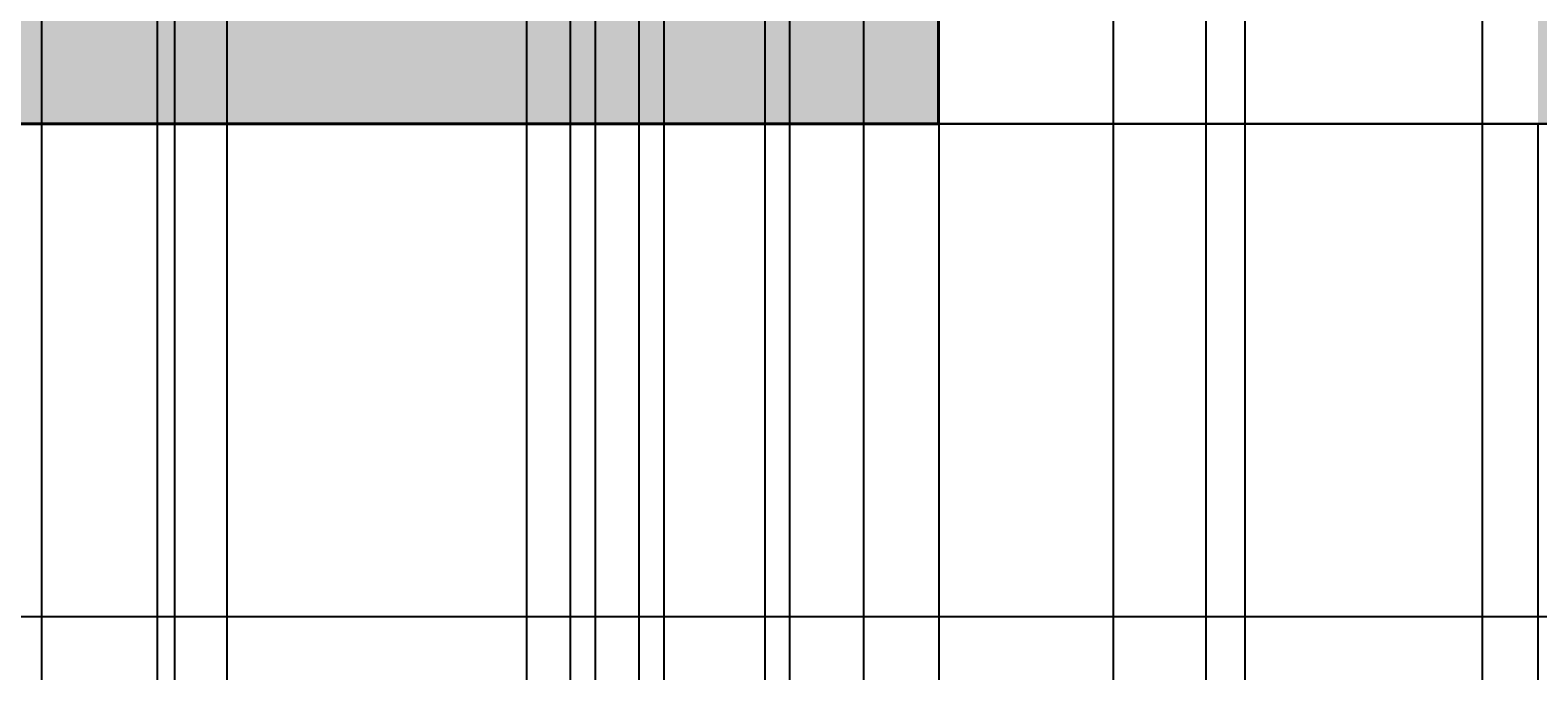
# Model space of a CAD drawing. Units: inches. Extents: x 818 to 1898, y 976 to 2364.
# Tile 35 of 96: x 1391 to 1512, y 1643 to 1695. Entities that reach past the tile are written whole.
import ezdxf

# ---------------------------------------------------------------- set-up
doc = ezdxf.new("R2010")
doc.units = ezdxf.units.IN
doc.header["$LTSCALE"] = 5
doc.header["$MEASUREMENT"] = 0
doc.layers.add('A-ANNO-DIMS', color=2, linetype='Continuous', lineweight=18)
doc.layers.add('A-WALL', color=7, linetype='Continuous', lineweight=40)
doc.layers.add('A-WALL-PATT', color=251, linetype='Continuous', lineweight=13, true_color=0x636466)
doc.styles.get("Standard").update_dxf_attribs({"font": 'arial.ttf'})
doc.dimstyles.get("Standard").update_dxf_attribs({"dimtxt": 0.18, "dimasz": 0.18, "dimexe": 0.18, "dimexo": 0.0625, "dimgap": 0.09, "dimtad": 0, "dimtih": 1, "dimtoh": 1, "dimdec": 4, "dimzin": 0, "dimdsep": 46, "dimtxsty": 'Standard', "dimcen": 0.09, "dimadec": 0, "dimazin": 0, "dimtfac": 1, "dimtdec": 4, "dimtofl": 0, "dimtmove": 0, "dimatfit": 3, "dimfxl": 1, "dimtolj": 1, "dimtzin": 0, "dimarcsym": 0})

# ---------------------------------------------------------------- blocks, each defined once
blk = doc.blocks.new('*D61')
at = {"layer": 'A-ANNO-DIMS', "color": 0, "lineweight": -2, "ltscale": 5, "transparency": 16777216}
for p, q in [((1071.73, 1203.03), (1071.73, 2363.87)), ((1071.91, 2363.69), (1250.94, 2363.69)), ((1430.55, 2363.69), (1251.51, 2363.69)), ((1430.73, 1203.03), (1430.73, 2363.87))]:
    blk.add_line(p, q, dxfattribs=at)
at = {"layer": 'A-ANNO-DIMS', "color": 0, "ltscale": 5, "transparency": 16777216}
for points in [[(1071.91, 2363.72), (1071.91, 2363.66), (1071.73, 2363.69)], [(1430.55, 2363.72), (1430.55, 2363.66), (1430.73, 2363.69)]]:
    blk.add_solid(points, dxfattribs=at)
at = {"layer": 'Defpoints', "color": 0, "ltscale": 5, "transparency": 16777216}
for p in [(1430.73, 2363.69), (1071.73, 1202.96), (1430.73, 1202.96)]:
    blk.add_point(p, dxfattribs=at)
at = {"layer": 'A-ANNO-DIMS', "color": 0, "ltscale": 5, "transparency": 16777216, "insert": (1251.23, 2363.69), "char_height": 0.18, "attachment_point": 5}
blk.add_mtext('\\A1;359', dxfattribs=at)
blk = doc.blocks.new('*D64')
at = {"layer": 'A-ANNO-DIMS', "color": 0, "lineweight": -2, "ltscale": 5, "transparency": 16777216}
for p, q in [((1197.73, 1501.14), (1197.73, 2363.87)), ((1197.91, 2363.69), (1313.93, 2363.69)), ((1430.55, 2363.69), (1314.52, 2363.69)), ((1430.73, 1501.14), (1430.73, 2363.87))]:
    blk.add_line(p, q, dxfattribs=at)
at = {"layer": 'A-ANNO-DIMS', "color": 0, "ltscale": 5, "transparency": 16777216}
for points in [[(1197.91, 2363.72), (1197.91, 2363.66), (1197.73, 2363.69)], [(1430.55, 2363.72), (1430.55, 2363.66), (1430.73, 2363.69)]]:
    blk.add_solid(points, dxfattribs=at)
at = {"layer": 'Defpoints', "color": 0, "ltscale": 5, "transparency": 16777216}
for p in [(1430.73, 2363.69), (1197.73, 1501.08), (1430.73, 1501.08)]:
    blk.add_point(p, dxfattribs=at)
at = {"layer": 'A-ANNO-DIMS', "color": 0, "ltscale": 5, "transparency": 16777216, "insert": (1314.23, 2363.69), "char_height": 0.18, "attachment_point": 5}
blk.add_mtext('\\A1;233', dxfattribs=at)
blk = doc.blocks.new('*D98')
at = {"layer": 'A-ANNO-DIMS', "color": 0, "lineweight": -2, "ltscale": 5, "transparency": 16777216}
for p, q in [((1338.54, 1071.12), (1338.54, 2363.87)), ((1338.72, 2363.69), (1364.81, 2363.69)), ((1391.7, 2363.69), (1365.6, 2363.69)), ((1391.88, 1071.12), (1391.88, 2363.87))]:
    blk.add_line(p, q, dxfattribs=at)
at = {"layer": 'A-ANNO-DIMS', "color": 0, "ltscale": 5, "transparency": 16777216}
for points in [[(1338.72, 2363.72), (1338.72, 2363.66), (1338.54, 2363.69)], [(1391.7, 2363.72), (1391.7, 2363.66), (1391.88, 2363.69)]]:
    blk.add_solid(points, dxfattribs=at)
at = {"layer": 'Defpoints', "color": 0, "ltscale": 5, "transparency": 16777216}
for p in [(1391.88, 2363.69), (1338.54, 1071.06), (1391.88, 1071.06)]:
    blk.add_point(p, dxfattribs=at)
at = {"layer": 'A-ANNO-DIMS', "color": 0, "ltscale": 5, "transparency": 16777216, "insert": (1365.21, 2363.69), "char_height": 0.18, "attachment_point": 5}
blk.add_mtext('\\A1;53.33', dxfattribs=at)
blk = doc.blocks.new('*D99')
at = {"layer": 'A-ANNO-DIMS', "color": 0, "lineweight": -2, "ltscale": 5, "transparency": 16777216}
for p, q in [((1391.88, 1071.12), (1391.88, 2363.87)), ((1392.06, 2363.69), (1420.45, 2363.69)), ((1449.64, 2363.69), (1421.24, 2363.69)), ((1449.82, 1071.12), (1449.82, 2363.87))]:
    blk.add_line(p, q, dxfattribs=at)
at = {"layer": 'A-ANNO-DIMS', "color": 0, "ltscale": 5, "transparency": 16777216}
for points in [[(1392.06, 2363.72), (1392.06, 2363.66), (1391.88, 2363.69)], [(1449.64, 2363.72), (1449.64, 2363.66), (1449.82, 2363.69)]]:
    blk.add_solid(points, dxfattribs=at)
at = {"layer": 'Defpoints', "color": 0, "ltscale": 5, "transparency": 16777216}
for p in [(1449.82, 2363.69), (1391.88, 1071.06), (1449.82, 1071.06)]:
    blk.add_point(p, dxfattribs=at)
at = {"layer": 'A-ANNO-DIMS', "color": 0, "ltscale": 5, "transparency": 16777216, "insert": (1420.85, 2363.69), "char_height": 0.18, "attachment_point": 5}
blk.add_mtext('\\A1;57.94', dxfattribs=at)
blk = doc.blocks.new('*D100')
at = {"layer": 'A-ANNO-DIMS', "color": 0, "lineweight": -2, "ltscale": 5, "transparency": 16777216}
for p, q in [((1449.82, 1071.12), (1449.82, 2363.87)), ((1450, 2363.69), (1478.17, 2363.69)), ((1507.12, 2363.69), (1478.95, 2363.69)), ((1507.3, 1071.12), (1507.3, 2363.87))]:
    blk.add_line(p, q, dxfattribs=at)
at = {"layer": 'A-ANNO-DIMS', "color": 0, "ltscale": 5, "transparency": 16777216}
for points in [[(1450, 2363.72), (1450, 2363.66), (1449.82, 2363.69)], [(1507.12, 2363.72), (1507.12, 2363.66), (1507.3, 2363.69)]]:
    blk.add_solid(points, dxfattribs=at)
at = {"layer": 'Defpoints', "color": 0, "ltscale": 5, "transparency": 16777216}
for p in [(1507.3, 2363.69), (1449.82, 1071.06), (1507.3, 1071.06)]:
    blk.add_point(p, dxfattribs=at)
at = {"layer": 'A-ANNO-DIMS', "color": 0, "ltscale": 5, "transparency": 16777216, "insert": (1478.56, 2363.69), "char_height": 0.18, "attachment_point": 5}
blk.add_mtext('\\A1;57.48', dxfattribs=at)
blk = doc.blocks.new('*D101')
at = {"layer": 'A-ANNO-DIMS', "color": 0, "lineweight": -2, "ltscale": 5, "transparency": 16777216}
for p, q in [((1507.3, 1071.12), (1507.3, 2363.87)), ((1507.48, 2363.69), (1536, 2363.69)), ((1565.3, 2363.69), (1536.78, 2363.69)), ((1565.48, 1071.12), (1565.48, 2363.87))]:
    blk.add_line(p, q, dxfattribs=at)
at = {"layer": 'A-ANNO-DIMS', "color": 0, "ltscale": 5, "transparency": 16777216}
for points in [[(1507.48, 2363.72), (1507.48, 2363.66), (1507.3, 2363.69)], [(1565.3, 2363.72), (1565.3, 2363.66), (1565.48, 2363.69)]]:
    blk.add_solid(points, dxfattribs=at)
at = {"layer": 'Defpoints', "color": 0, "ltscale": 5, "transparency": 16777216}
for p in [(1565.48, 2363.69), (1507.3, 1071.06), (1565.48, 1071.06)]:
    blk.add_point(p, dxfattribs=at)
at = {"layer": 'A-ANNO-DIMS', "color": 0, "ltscale": 5, "transparency": 16777216, "insert": (1536.39, 2363.69), "char_height": 0.18, "attachment_point": 5}
blk.add_mtext('\\A1;58.19', dxfattribs=at)
blk = doc.blocks.new('*D119')
at = {"layer": 'A-ANNO-DIMS', "color": 0, "lineweight": -2, "ltscale": 5, "transparency": 16777216}
for p, q in [((1766.29, 1716.99), (818.03, 1716.99)), ((818.21, 1716.81), (818.21, 1672.43)), ((818.21, 1627.69), (818.21, 1672.06)), ((1766.29, 1627.51), (818.03, 1627.51))]:
    blk.add_line(p, q, dxfattribs=at)
at = {"layer": 'A-ANNO-DIMS', "color": 0, "ltscale": 5, "transparency": 16777216}
for points in [[(818.18, 1716.81), (818.24, 1716.81), (818.21, 1716.99)], [(818.18, 1627.69), (818.24, 1627.69), (818.21, 1627.51)]]:
    blk.add_solid(points, dxfattribs=at)
at = {"layer": 'Defpoints', "color": 0, "ltscale": 5, "transparency": 16777216}
for p in [(818.21, 1716.99), (1766.35, 1716.99), (1766.35, 1627.51)]:
    blk.add_point(p, dxfattribs=at)
at = {"layer": 'A-ANNO-DIMS', "color": 0, "ltscale": 5, "transparency": 16777216, "insert": (818.21, 1672.25), "char_height": 0.18, "attachment_point": 5}
blk.add_mtext('\\A1;89.48', dxfattribs=at)
blk = doc.blocks.new('*D159')
at = {"layer": 'A-ANNO-DIMS', "color": 0, "lineweight": -2, "ltscale": 5, "transparency": 16777216}
for p, q in [((1206.73, 1687.02), (1206.73, 975.66)), ((1463.73, 1687.02), (1463.73, 975.66)), ((1206.91, 975.84), (1334.93, 975.84)), ((1463.55, 975.84), (1335.52, 975.84))]:
    blk.add_line(p, q, dxfattribs=at)
at = {"layer": 'A-ANNO-DIMS', "color": 0, "ltscale": 5, "transparency": 16777216}
for points in [[(1206.91, 975.87), (1206.91, 975.81), (1206.73, 975.84)], [(1463.55, 975.87), (1463.55, 975.81), (1463.73, 975.84)]]:
    blk.add_solid(points, dxfattribs=at)
at = {"layer": 'Defpoints', "color": 0, "ltscale": 5, "transparency": 16777216}
for p in [(1206.73, 1687.08), (1463.73, 1687.08), (1463.73, 975.84)]:
    blk.add_point(p, dxfattribs=at)
at = {"layer": 'A-ANNO-DIMS', "color": 0, "ltscale": 5, "transparency": 16777216, "insert": (1335.23, 975.84), "char_height": 0.18, "attachment_point": 5}
blk.add_mtext('\\A1;257', dxfattribs=at)
blk = doc.blocks.new('*D160')
at = {"layer": 'A-ANNO-DIMS', "color": 0, "lineweight": -2, "ltscale": 5, "transparency": 16777216}
for p, q in [((1463.73, 1687.02), (1463.73, 975.66)), ((1511.73, 1687.02), (1511.73, 975.66)), ((1463.91, 975.84), (1487.5, 975.84)), ((1511.55, 975.84), (1487.95, 975.84))]:
    blk.add_line(p, q, dxfattribs=at)
at = {"layer": 'A-ANNO-DIMS', "color": 0, "ltscale": 5, "transparency": 16777216}
for points in [[(1463.91, 975.87), (1463.91, 975.81), (1463.73, 975.84)], [(1511.55, 975.87), (1511.55, 975.81), (1511.73, 975.84)]]:
    blk.add_solid(points, dxfattribs=at)
at = {"layer": 'Defpoints', "color": 0, "ltscale": 5, "transparency": 16777216}
for p in [(1463.73, 1687.08), (1511.73, 1687.08), (1511.73, 975.84)]:
    blk.add_point(p, dxfattribs=at)
at = {"layer": 'A-ANNO-DIMS', "color": 0, "ltscale": 5, "transparency": 16777216, "insert": (1487.73, 975.84), "char_height": 0.18, "attachment_point": 5}
blk.add_mtext('\\A1;48', dxfattribs=at)
blk = doc.blocks.new('*D166')
at = {"layer": 'A-ANNO-DIMS', "color": 0, "lineweight": -2, "ltscale": 5, "transparency": 16777216}
for p, q in [((1401.15, 1510.14), (1401.15, 2363.87)), ((1401.33, 2363.69), (1415.54, 2363.69)), ((1430.55, 2363.69), (1416.33, 2363.69)), ((1430.73, 1510.14), (1430.73, 2363.87))]:
    blk.add_line(p, q, dxfattribs=at)
at = {"layer": 'A-ANNO-DIMS', "color": 0, "ltscale": 5, "transparency": 16777216}
for points in [[(1401.33, 2363.72), (1401.33, 2363.66), (1401.15, 2363.69)], [(1430.55, 2363.72), (1430.55, 2363.66), (1430.73, 2363.69)]]:
    blk.add_solid(points, dxfattribs=at)
at = {"layer": 'Defpoints', "color": 0, "ltscale": 5, "transparency": 16777216}
for p in [(1430.73, 2363.69), (1401.15, 1510.08), (1430.73, 1510.08)]:
    blk.add_point(p, dxfattribs=at)
at = {"layer": 'A-ANNO-DIMS', "color": 0, "ltscale": 5, "transparency": 16777216, "insert": (1415.94, 2363.69), "char_height": 0.18, "attachment_point": 5}
blk.add_mtext('\\A1;29.58', dxfattribs=at)
blk = doc.blocks.new('*D169')
at = {"layer": 'A-ANNO-DIMS', "color": 0, "lineweight": -2, "ltscale": 5, "transparency": 16777216}
for p, q in [((1441.73, 1600.14), (1441.73, 2363.87)), ((1441.91, 2363.69), (1459.51, 2363.69)), ((1477.55, 2363.69), (1459.94, 2363.69)), ((1477.73, 1600.14), (1477.73, 2363.87))]:
    blk.add_line(p, q, dxfattribs=at)
at = {"layer": 'A-ANNO-DIMS', "color": 0, "ltscale": 5, "transparency": 16777216}
for points in [[(1441.91, 2363.72), (1441.91, 2363.66), (1441.73, 2363.69)], [(1477.55, 2363.72), (1477.55, 2363.66), (1477.73, 2363.69)]]:
    blk.add_solid(points, dxfattribs=at)
at = {"layer": 'Defpoints', "color": 0, "ltscale": 5, "transparency": 16777216}
for p in [(1477.73, 2363.69), (1441.73, 1600.08), (1477.73, 1600.08)]:
    blk.add_point(p, dxfattribs=at)
at = {"layer": 'A-ANNO-DIMS', "color": 0, "ltscale": 5, "transparency": 16777216, "insert": (1459.73, 2363.69), "char_height": 0.18, "attachment_point": 5}
blk.add_mtext('\\A1;36', dxfattribs=at)
blk = doc.blocks.new('*D176')
at = {"layer": 'A-ANNO-DIMS', "color": 0, "lineweight": -2, "ltscale": 5, "transparency": 16777216}
for p, q in [((1559.66, 1687.08), (818.03, 1687.08)), ((818.21, 1686.9), (818.21, 1667.51)), ((818.21, 1647.76), (818.21, 1667.15)), ((1559.66, 1647.58), (818.03, 1647.58))]:
    blk.add_line(p, q, dxfattribs=at)
at = {"layer": 'A-ANNO-DIMS', "color": 0, "ltscale": 5, "transparency": 16777216}
for points in [[(818.18, 1686.9), (818.24, 1686.9), (818.21, 1687.08)], [(818.18, 1647.76), (818.24, 1647.76), (818.21, 1647.58)]]:
    blk.add_solid(points, dxfattribs=at)
at = {"layer": 'Defpoints', "color": 0, "ltscale": 5, "transparency": 16777216}
for p in [(1559.73, 1687.08), (818.21, 1647.58), (1559.73, 1647.58)]:
    blk.add_point(p, dxfattribs=at)
at = {"layer": 'A-ANNO-DIMS', "color": 0, "ltscale": 5, "transparency": 16777216, "insert": (818.21, 1667.33), "char_height": 0.18, "attachment_point": 5}
blk.add_mtext('\\A1;39.5', dxfattribs=at)
blk = doc.blocks.new('*D182')
at = {"layer": 'A-ANNO-DIMS', "color": 0, "lineweight": -2, "ltscale": 5, "transparency": 16777216}
for p, q in [((1463.73, 1687.02), (1463.73, 975.66)), ((1559.73, 1687.02), (1559.73, 975.66)), ((1463.91, 975.84), (1511.51, 975.84)), ((1559.55, 975.84), (1511.94, 975.84))]:
    blk.add_line(p, q, dxfattribs=at)
at = {"layer": 'A-ANNO-DIMS', "color": 0, "ltscale": 5, "transparency": 16777216}
for points in [[(1463.91, 975.87), (1463.91, 975.81), (1463.73, 975.84)], [(1559.55, 975.87), (1559.55, 975.81), (1559.73, 975.84)]]:
    blk.add_solid(points, dxfattribs=at)
at = {"layer": 'Defpoints', "color": 0, "ltscale": 5, "transparency": 16777216}
for p in [(1463.73, 1687.08), (1559.73, 1687.08), (1559.73, 975.84)]:
    blk.add_point(p, dxfattribs=at)
at = {"layer": 'A-ANNO-DIMS', "color": 0, "ltscale": 5, "transparency": 16777216, "insert": (1511.73, 975.84), "char_height": 0.18, "attachment_point": 5}
blk.add_mtext('\\A1;96', dxfattribs=at)
blk = doc.blocks.new('*D191')
at = {"layer": 'A-ANNO-DIMS', "color": 0, "lineweight": -2, "ltscale": 5, "transparency": 16777216}
for p, q in [((1434.23, 1409.11), (1434.23, 2363.87)), ((1434.41, 2363.69), (1435.08, 2363.69)), ((1436.05, 2363.69), (1435.37, 2363.69)), ((1436.23, 1409.11), (1436.23, 2363.87))]:
    blk.add_line(p, q, dxfattribs=at)
at = {"layer": 'A-ANNO-DIMS', "color": 0, "ltscale": 5, "transparency": 16777216}
for points in [[(1434.41, 2363.72), (1434.41, 2363.66), (1434.23, 2363.69)], [(1436.05, 2363.72), (1436.05, 2363.66), (1436.23, 2363.69)]]:
    blk.add_solid(points, dxfattribs=at)
at = {"layer": 'Defpoints', "color": 0, "ltscale": 5, "transparency": 16777216}
for p in [(1436.23, 2363.69), (1434.23, 1409.05), (1436.23, 1409.05)]:
    blk.add_point(p, dxfattribs=at)
at = {"layer": 'A-ANNO-DIMS', "color": 0, "ltscale": 5, "transparency": 16777216, "insert": (1435.23, 2363.69), "char_height": 0.18, "attachment_point": 5}
blk.add_mtext('\\A1;2', dxfattribs=at)
blk = doc.blocks.new('*D196')
at = {"layer": 'A-ANNO-DIMS', "color": 0, "lineweight": -2, "ltscale": 5, "transparency": 16777216}
for p, q in [((1439.73, 1526.73), (1439.73, 2363.87)), ((1439.91, 2363.69), (1448.51, 2363.69)), ((1457.55, 2363.69), (1448.94, 2363.69)), ((1457.73, 1526.73), (1457.73, 2363.87))]:
    blk.add_line(p, q, dxfattribs=at)
at = {"layer": 'A-ANNO-DIMS', "color": 0, "ltscale": 5, "transparency": 16777216}
for points in [[(1439.91, 2363.72), (1439.91, 2363.66), (1439.73, 2363.69)], [(1457.55, 2363.72), (1457.55, 2363.66), (1457.73, 2363.69)]]:
    blk.add_solid(points, dxfattribs=at)
at = {"layer": 'Defpoints', "color": 0, "ltscale": 5, "transparency": 16777216}
for p in [(1457.73, 2363.69), (1439.73, 1526.67), (1457.73, 1526.67)]:
    blk.add_point(p, dxfattribs=at)
at = {"layer": 'A-ANNO-DIMS', "color": 0, "ltscale": 5, "transparency": 16777216, "insert": (1448.73, 2363.69), "char_height": 0.18, "attachment_point": 5}
blk.add_mtext('\\A1;18', dxfattribs=at)
blk = doc.blocks.new('*D214')
at = {"layer": 'A-ANNO-DIMS', "color": 0, "lineweight": -2, "ltscale": 5, "transparency": 16777216}
for p, q in [((1511.73, 1687.02), (1511.73, 975.66)), ((1714.73, 1687.02), (1714.73, 975.66)), ((1511.91, 975.84), (1612.93, 975.84)), ((1714.55, 975.84), (1613.52, 975.84))]:
    blk.add_line(p, q, dxfattribs=at)
at = {"layer": 'A-ANNO-DIMS', "color": 0, "ltscale": 5, "transparency": 16777216}
for points in [[(1511.91, 975.87), (1511.91, 975.81), (1511.73, 975.84)], [(1714.55, 975.87), (1714.55, 975.81), (1714.73, 975.84)]]:
    blk.add_solid(points, dxfattribs=at)
at = {"layer": 'Defpoints', "color": 0, "ltscale": 5, "transparency": 16777216}
for p in [(1511.73, 1687.08), (1714.73, 1687.08), (1714.73, 975.84)]:
    blk.add_point(p, dxfattribs=at)
at = {"layer": 'A-ANNO-DIMS', "color": 0, "ltscale": 5, "transparency": 16777216, "insert": (1613.23, 975.84), "char_height": 0.18, "attachment_point": 5}
blk.add_mtext('\\A1;203', dxfattribs=at)
blk = doc.blocks.new('*D215')
at = {"layer": 'A-ANNO-DIMS', "color": 0, "lineweight": -2, "ltscale": 5, "transparency": 16777216}
for p, q in [((1590.66, 1876.08), (818.03, 1876.08)), ((818.21, 1875.9), (818.21, 1781.76)), ((818.21, 1687.26), (818.21, 1781.4)), ((1511.66, 1687.08), (818.03, 1687.08))]:
    blk.add_line(p, q, dxfattribs=at)
at = {"layer": 'A-ANNO-DIMS', "color": 0, "ltscale": 5, "transparency": 16777216}
for points in [[(818.18, 1875.9), (818.24, 1875.9), (818.21, 1876.08)], [(818.18, 1687.26), (818.24, 1687.26), (818.21, 1687.08)]]:
    blk.add_solid(points, dxfattribs=at)
at = {"layer": 'Defpoints', "color": 0, "ltscale": 5, "transparency": 16777216}
for p in [(818.21, 1876.08), (1590.73, 1876.08), (1511.73, 1687.08)]:
    blk.add_point(p, dxfattribs=at)
at = {"layer": 'A-ANNO-DIMS', "color": 0, "ltscale": 5, "transparency": 16777216, "insert": (818.21, 1781.58), "char_height": 0.18, "attachment_point": 5}
blk.add_mtext('\\A1;189', dxfattribs=at)
blk = doc.blocks.new('*D231')
at = {"layer": 'A-ANNO-DIMS', "color": 0, "lineweight": -2, "ltscale": 5, "transparency": 16777216}
for p, q in [((1303.93, 1952.98), (1303.93, 975.66)), ((1402.52, 1952.98), (1402.52, 975.66)), ((1304.11, 975.84), (1352.83, 975.84)), ((1402.34, 975.84), (1353.62, 975.84))]:
    blk.add_line(p, q, dxfattribs=at)
at = {"layer": 'A-ANNO-DIMS', "color": 0, "ltscale": 5, "transparency": 16777216}
for points in [[(1304.11, 975.87), (1304.11, 975.81), (1303.93, 975.84)], [(1402.34, 975.87), (1402.34, 975.81), (1402.52, 975.84)]]:
    blk.add_solid(points, dxfattribs=at)
at = {"layer": 'Defpoints', "color": 0, "ltscale": 5, "transparency": 16777216}
for p in [(1303.93, 1953.04), (1402.52, 1953.04), (1402.52, 975.84)]:
    blk.add_point(p, dxfattribs=at)
at = {"layer": 'A-ANNO-DIMS', "color": 0, "ltscale": 5, "transparency": 16777216, "insert": (1353.22, 975.84), "char_height": 0.18, "attachment_point": 5}
blk.add_mtext('\\A1;98.59', dxfattribs=at)
blk = doc.blocks.new('*D242')
at = {"layer": 'A-ANNO-DIMS', "color": 0, "lineweight": -2, "ltscale": 5, "transparency": 16777216}
for p, q in [((1488.26, 1948.6), (1488.26, 975.66)), ((1513.23, 1948.6), (1513.23, 975.66)), ((1488.44, 975.84), (1500.35, 975.84)), ((1513.05, 975.84), (1501.14, 975.84))]:
    blk.add_line(p, q, dxfattribs=at)
at = {"layer": 'A-ANNO-DIMS', "color": 0, "ltscale": 5, "transparency": 16777216}
for points in [[(1488.44, 975.87), (1488.44, 975.81), (1488.26, 975.84)], [(1513.05, 975.87), (1513.05, 975.81), (1513.23, 975.84)]]:
    blk.add_solid(points, dxfattribs=at)
at = {"layer": 'Defpoints', "color": 0, "ltscale": 5, "transparency": 16777216}
for p in [(1488.26, 1948.66), (1513.23, 1948.66), (1513.23, 975.84)]:
    blk.add_point(p, dxfattribs=at)
at = {"layer": 'A-ANNO-DIMS', "color": 0, "ltscale": 5, "transparency": 16777216, "insert": (1500.74, 975.84), "char_height": 0.18, "attachment_point": 5}
blk.add_mtext('\\A1;24.97', dxfattribs=at)
blk = doc.blocks.new('*D243')
at = {"layer": 'A-ANNO-DIMS', "color": 0, "lineweight": -2, "ltscale": 5, "transparency": 16777216}
for p, q in [((1451.77, 2020.02), (1451.77, 975.66)), ((1590.73, 2020.02), (1590.73, 975.66)), ((1451.95, 975.84), (1520.79, 975.84)), ((1590.55, 975.84), (1521.7, 975.84))]:
    blk.add_line(p, q, dxfattribs=at)
at = {"layer": 'A-ANNO-DIMS', "color": 0, "ltscale": 5, "transparency": 16777216}
for points in [[(1451.95, 975.87), (1451.95, 975.81), (1451.77, 975.84)], [(1590.55, 975.87), (1590.55, 975.81), (1590.73, 975.84)]]:
    blk.add_solid(points, dxfattribs=at)
at = {"layer": 'Defpoints', "color": 0, "ltscale": 5, "transparency": 16777216}
for p in [(1451.77, 2020.08), (1590.73, 2020.08), (1590.73, 975.84)]:
    blk.add_point(p, dxfattribs=at)
at = {"layer": 'A-ANNO-DIMS', "color": 0, "ltscale": 5, "transparency": 16777216, "insert": (1521.25, 975.84), "char_height": 0.18, "attachment_point": 5}
blk.add_mtext('\\A1;138.96', dxfattribs=at)
blk = doc.blocks.new('*D253')
at = {"layer": 'A-ANNO-DIMS', "color": 0, "lineweight": -2, "ltscale": 5, "transparency": 16777216}
for p, q in [((1485.12, 2053.02), (1485.12, 975.66)), ((1538.52, 2053.02), (1538.52, 975.66)), ((1485.3, 975.84), (1511.42, 975.84)), ((1538.34, 975.84), (1512.21, 975.84))]:
    blk.add_line(p, q, dxfattribs=at)
at = {"layer": 'A-ANNO-DIMS', "color": 0, "ltscale": 5, "transparency": 16777216}
for points in [[(1485.3, 975.87), (1485.3, 975.81), (1485.12, 975.84)], [(1538.34, 975.87), (1538.34, 975.81), (1538.52, 975.84)]]:
    blk.add_solid(points, dxfattribs=at)
at = {"layer": 'Defpoints', "color": 0, "ltscale": 5, "transparency": 16777216}
for p in [(1485.12, 2053.08), (1538.52, 2053.08), (1538.52, 975.84)]:
    blk.add_point(p, dxfattribs=at)
at = {"layer": 'A-ANNO-DIMS', "color": 0, "ltscale": 5, "transparency": 16777216, "insert": (1511.82, 975.84), "char_height": 0.18, "attachment_point": 5}
blk.add_mtext('\\A1;53.39', dxfattribs=at)
blk = doc.blocks.new('*D273')
at = {"layer": 'A-ANNO-DIMS', "color": 0, "lineweight": -2, "ltscale": 5, "transparency": 16777216}
for p, q in [((1406.73, 1587.48), (1406.73, 2363.87)), ((1406.91, 2363.69), (1418.51, 2363.69)), ((1430.55, 2363.69), (1418.95, 2363.69)), ((1430.73, 1587.48), (1430.73, 2363.87))]:
    blk.add_line(p, q, dxfattribs=at)
at = {"layer": 'A-ANNO-DIMS', "color": 0, "ltscale": 5, "transparency": 16777216}
for points in [[(1406.91, 2363.72), (1406.91, 2363.66), (1406.73, 2363.69)], [(1430.55, 2363.72), (1430.55, 2363.66), (1430.73, 2363.69)]]:
    blk.add_solid(points, dxfattribs=at)
at = {"layer": 'Defpoints', "color": 0, "ltscale": 5, "transparency": 16777216}
for p in [(1430.73, 2363.69), (1406.73, 1587.42), (1430.73, 1587.42)]:
    blk.add_point(p, dxfattribs=at)
at = {"layer": 'A-ANNO-DIMS', "color": 0, "ltscale": 5, "transparency": 16777216, "insert": (1418.73, 2363.69), "char_height": 0.18, "attachment_point": 5}
blk.add_mtext('\\A1;24', dxfattribs=at)
blk = doc.blocks.new('*D282')
at = {"layer": 'A-ANNO-DIMS', "color": 0, "lineweight": -2, "ltscale": 5, "transparency": 16777216}
for p, q in [((1422.08, 2081.19), (1897.92, 2081.19)), ((1897.74, 2081.01), (1897.74, 1884.32)), ((1897.74, 1687.26), (1897.74, 1883.95)), ((1463.79, 1687.08), (1897.92, 1687.08))]:
    blk.add_line(p, q, dxfattribs=at)
at = {"layer": 'A-ANNO-DIMS', "color": 0, "ltscale": 5, "transparency": 16777216}
for points in [[(1897.71, 2081.01), (1897.77, 2081.01), (1897.74, 2081.19)], [(1897.71, 1687.26), (1897.77, 1687.26), (1897.74, 1687.08)]]:
    blk.add_solid(points, dxfattribs=at)
at = {"layer": 'Defpoints', "color": 0, "ltscale": 5, "transparency": 16777216}
for p in [(1422.02, 2081.19), (1897.74, 2081.19), (1463.73, 1687.08)]:
    blk.add_point(p, dxfattribs=at)
at = {"layer": 'A-ANNO-DIMS', "color": 0, "ltscale": 5, "transparency": 16777216, "insert": (1897.74, 1884.13), "char_height": 0.18, "attachment_point": 5}
blk.add_mtext('\\A1;394.1', dxfattribs=at)
blk = doc.blocks.new('*D291')
at = {"layer": 'A-ANNO-DIMS', "color": 0, "lineweight": -2, "ltscale": 5, "transparency": 16777216}
for p, q in [((1206.79, 1687.08), (1897.92, 1687.08)), ((1897.74, 1686.9), (1897.74, 1647.61)), ((1897.74, 1607.95), (1897.74, 1647.24)), ((1318.96, 1607.77), (1897.92, 1607.77))]:
    blk.add_line(p, q, dxfattribs=at)
at = {"layer": 'A-ANNO-DIMS', "color": 0, "ltscale": 5, "transparency": 16777216}
for points in [[(1897.71, 1686.9), (1897.77, 1686.9), (1897.74, 1687.08)], [(1897.71, 1607.95), (1897.77, 1607.95), (1897.74, 1607.77)]]:
    blk.add_solid(points, dxfattribs=at)
at = {"layer": 'Defpoints', "color": 0, "ltscale": 5, "transparency": 16777216}
for p in [(1206.73, 1687.08), (1897.74, 1687.08), (1318.89, 1607.77)]:
    blk.add_point(p, dxfattribs=at)
at = {"layer": 'A-ANNO-DIMS', "color": 0, "ltscale": 5, "transparency": 16777216, "insert": (1897.74, 1647.42), "char_height": 0.18, "attachment_point": 5}
blk.add_mtext('\\A1;79.3', dxfattribs=at)

msp = doc.modelspace()

# ---------------------------------------------------------------- hatches: boundary and pattern name
at = {"layer": 'A-WALL-PATT', "ltscale": 5}
h = msp.add_hatch(color=256, dxfattribs=at)
h.dxf.hatch_style = 1
h.paths.add_polyline_path([(1267.7252, 1928.9218), (1258.7252, 1928.9218), (1258.7252, 1913.6401), (1250.3029, 1913.6401), (1250.3029, 1878.3919), (1258.7252, 1878.3919), (1258.7252, 1862.9652), (1267.7252, 1862.9652)])
h.paths.add_polyline_path([(1267.7252, 1814.9652), (1258.7252, 1814.9652), (1258.7252, 1755.3321), (1267.7252, 1755.3321)])
h.paths.add_polyline_path([(1463.7251, 1696.0782), (1267.7252, 1696.0782), (1267.7252, 1707.3321), (1258.7252, 1707.3321), (1258.7252, 1700.0782), (1251.9333, 1700.0782), (1251.9333, 1687.0782), (1463.7251, 1687.0782)])
h.paths.add_polyline_path([(1714.7251, 1717.3178), (1705.7252, 1717.3178), (1705.7252, 1696.0782), (1599.7252, 1696.0782), (1599.7252, 1790.0782), (1705.7252, 1790.0782), (1705.7252, 1785.6125), (1714.7251, 1785.6125), (1714.7251, 1827.2125), (1705.7252, 1827.2125), (1705.7252, 1802.0782), (1599.7252, 1802.0782), (1599.7252, 1867.0782), (1705.7252, 1867.0782), (1705.7252, 1857.2125), (1714.7251, 1857.2125), (1714.7251, 1930.0316), (1741.8409, 1930.0316), (1741.8409, 1935.0316), (1714.7251, 1935.0316), (1714.7251, 1957.0338), (1741.8409, 1957.0338), (1741.8409, 1962.0338), (1714.7251, 1962.0338), (1705.7252, 1962.0338), (1705.7252, 1948.0782), (1599.7252, 1948.0782), (1599.7252, 1981.0782), (1590.7251, 1981.0782), (1590.7251, 1941.0782), (1620.7252, 1941.0782), (1705.7252, 1941.0782), (1705.7252, 1876.0782), (1599.7252, 1876.0782), (1599.7252, 1911.0782), (1590.7251, 1911.0782), (1590.7251, 1876.0782), (1429.2252, 1876.0782), (1429.2252, 1867.0782), (1511.7251, 1867.0782), (1528.593, 1867.0782), (1595.7252, 1867.0782), (1595.7252, 1773.0782), (1520.7252, 1773.0782), (1520.7252, 1837.5823), (1532.593, 1837.5823), (1532.593, 1867.0782), (1528.593, 1867.0782), (1528.593, 1841.5823), (1511.7251, 1841.5823), (1511.7251, 1744.9714), (1520.7252, 1744.9714), (1520.7252, 1761.0782), (1595.7252, 1761.0782), (1595.7252, 1696.0782), (1520.7252, 1696.0782), (1520.7252, 1716.0454), (1511.7251, 1716.0454), (1511.7251, 1696.0782), (1511.7251, 1687.0782), (1714.7251, 1687.0782)])
h.paths.add_polyline_path([(1714.7251, 2053.0782), (1714.7251, 2081.1881), (1709.7252, 2081.1881), (1709.7252, 2053.0782), (1681.6446, 2053.0782), (1681.6446, 2081.1881), (1676.6446, 2081.1881), (1676.6446, 2053.0782), (1538.5155, 2053.0782), (1538.5155, 2044.0782), (1590.7251, 2044.0782), (1590.7251, 2011.0782), (1599.7252, 2011.0782), (1599.7252, 2044.0782), (1705.7252, 2044.0782), (1705.7252, 2014.5114), (1714.7251, 2014.5114)])
h.paths.add_polyline_path([(1485.1216, 2053.0782), (1422.02, 2053.0782), (1422.02, 2081.1881), (1413.02, 2081.1881), (1413.02, 2053.0782), (1399.6356, 2053.0782), (1399.6356, 2081.1881), (1390.6356, 2081.1881), (1390.6356, 2053.0782), (1388.0315, 2053.0782), (1388.0315, 2044.0782), (1416.2743, 2044.0782), (1485.1216, 2044.0782)])
h.paths.add_polyline_path([(1330.305, 2053.0782), (1258.7252, 2053.0782), (1258.7252, 2019.2871), (1267.7252, 2019.2871), (1267.7252, 2044.0782), (1330.305, 2044.0782)])
h.paths.add_polyline_path([(1258.7252, 2053.0782), (1214.6577, 2053.0782), (1214.6577, 2044.0782), (1258.7252, 2044.0782)])
h.paths.add_polyline_path([(1214.6577, 2053.0782), (1180.349, 2053.0782), (1180.349, 2044.0782), (1214.6577, 2044.0782)])
h.paths.add_polyline_path([(1714.7251, 1639.5782), (1741.8409, 1639.5782), (1741.8409, 1643.5782), (1714.7251, 1643.5782), (1714.7251, 1649.9029), (1705.7252, 1649.9029), (1705.7252, 1600.0782), (1477.7251, 1600.0782), (1477.7251, 1591.0782), (1520.7252, 1591.0782), (1616.7252, 1591.0782), (1616.7252, 1416.6857), (1622.7252, 1416.6857), (1622.7252, 1463.0782), (1624.7252, 1463.0782), (1624.7252, 1467.0782), (1622.7252, 1467.0782), (1622.7252, 1591.0782), (1705.7252, 1591.0782), (1705.7252, 1545.0782), (1714.7251, 1545.0782), (1741.8409, 1545.0782), (1741.8409, 1549.0782), (1714.7251, 1549.0782), (1714.7251, 1593.9175), (1737.8409, 1593.9175), (1737.8409, 1597.9175), (1714.7251, 1597.9175)])
h.paths.add_polyline_path([(1674.9024, 2060.7419), (1714.7045, 2060.7419), (1714.7045, 2073.1061), (1674.9024, 2073.1061)], flags=25)
h.paths.add_polyline_path([(1394.5468, 2061.6618), (1422.2344, 2061.6618), (1422.2344, 2074.0261), (1394.5468, 2074.0261)], flags=24)

# ---------------------------------------------------------------- linework, layer by layer
at = {"layer": 'A-WALL'}
for p in [(1463.7251, 1696.0782), (1206.7251, 1687.0782)]:
    msp.add_line(p, (1463.7251, 1687.0782), dxfattribs=at)

# ---------------------------------------------------------------- dimensions: what is measured, and where the dimension line sits
at = {"layer": 'A-ANNO-DIMS', "ltscale": 5}
for base, p1, p2, override, picture, middle in [((1430.7251, 2363.6929), (1071.7251, 1202.9642), (1430.7251, 1202.9642), {"dimdec": 0, "dimlfac": 1, "dimrnd": 0, "dimzin": 0, "dimdsep": 46, "dimlunit": 2}, '*D61', (1251.2251, 2363.6929)), ((1430.7251, 2363.6929), (1197.7251, 1501.0782), (1430.7251, 1501.0782), {"dimdec": 0, "dimlfac": 1, "dimrnd": 0, "dimzin": 0, "dimdsep": 46, "dimlunit": 2}, '*D64', (1314.2251, 2363.6929)), ((1391.8757, 2363.6929), (1338.5412, 1071.0552), (1391.8757, 1071.0552), {"dimdec": 2, "dimlfac": 1, "dimrnd": 0, "dimzin": 0, "dimdsep": 46, "dimlunit": 2}, '*D98', (1365.2084, 2363.6929)), ((1449.8196, 2363.6929), (1391.8757, 1071.0552), (1449.8196, 1071.0552), {"dimdec": 2, "dimlfac": 1, "dimrnd": 0, "dimzin": 0, "dimdsep": 46, "dimlunit": 2}, '*D99', (1420.8477, 2363.6929)), ((1430.7251, 2363.6929), (1401.1463, 1510.0782), (1430.7251, 1510.0782), {"dimdec": 2, "dimlfac": 1, "dimrnd": 0, "dimzin": 0, "dimdsep": 46, "dimlunit": 2}, '*D166', (1415.9357, 2363.6929)), ((1430.7251, 2363.6929), (1406.7251, 1587.4164), (1430.7251, 1587.4164), {"dimdec": 0, "dimlfac": 1, "dimrnd": 0, "dimzin": 0, "dimdsep": 46, "dimlunit": 2}, '*D273', (1418.7251, 2363.6929)), ((1436.2251, 2363.6929), (1434.2251, 1409.0522), (1436.2251, 1409.0522), {"dimdec": 0, "dimlfac": 1, "dimrnd": 0, "dimzin": 0, "dimdsep": 46, "dimlunit": 2}, '*D191', (1435.2251, 2363.6929)), ((1457.7251, 2363.6929), (1439.7251, 1526.6712), (1457.7251, 1526.6712), {"dimdec": 0, "dimlfac": 1, "dimrnd": 0, "dimzin": 0, "dimdsep": 46, "dimlunit": 2}, '*D196', (1448.7251, 2363.6929)), ((1477.7251, 2363.6929), (1441.7251, 1600.0782), (1477.7251, 1600.0782), {"dimdec": 0, "dimlfac": 1, "dimrnd": 0, "dimzin": 0, "dimdsep": 46, "dimlunit": 2}, '*D169', (1459.7251, 2363.6929)), ((1507.2982, 2363.6929), (1449.8196, 1071.0552), (1507.2982, 1071.0552), {"dimdec": 2, "dimlfac": 1, "dimrnd": 0, "dimzin": 0, "dimdsep": 46, "dimlunit": 2}, '*D100', (1478.5589, 2363.6929)), ((1565.4835, 2363.6929), (1507.2982, 1071.0552), (1565.4835, 1071.0552), {"dimdec": 2, "dimlfac": 1, "dimrnd": 0, "dimzin": 0, "dimdsep": 46, "dimlunit": 2}, '*D101', (1536.3908, 2363.6929)), ((1538.5155, 975.8433), (1485.1216, 2053.0782), (1538.5155, 2053.0782), {"dimdec": 2, "dimlfac": 1, "dimrnd": 0, "dimzin": 0, "dimdsep": 46, "dimlunit": 2}, '*D253', (1511.8185, 975.8433)), ((1590.7251, 975.8433), (1451.7698, 2020.0782), (1590.7251, 2020.0782), {"dimdec": 2, "dimlfac": 1, "dimrnd": 0, "dimzin": 0, "dimdsep": 46, "dimlunit": 2}, '*D243', (1521.2475, 975.8433)), ((1402.518, 975.8433), (1303.9314, 1953.0408), (1402.518, 1953.0408), {"dimdec": 2, "dimlfac": 1, "dimrnd": 0, "dimzin": 0, "dimdsep": 46, "dimlunit": 2}, '*D231', (1353.2247, 975.8433)), ((1513.2306, 975.8433), (1488.2586, 1948.6602), (1513.2306, 1948.6602), {"dimdec": 2, "dimlfac": 1, "dimrnd": 0, "dimzin": 0, "dimdsep": 46, "dimlunit": 2}, '*D242', (1500.7446, 975.8433)), ((1463.7251, 975.8433), (1206.7251, 1687.0782), (1463.7251, 1687.0782), {"dimdec": 0, "dimlfac": 1, "dimrnd": 0, "dimzin": 0, "dimdsep": 46, "dimlunit": 2}, '*D159', (1335.2251, 975.8433)), ((1511.7251, 975.8433), (1463.7251, 1687.0782), (1511.7251, 1687.0782), {"dimdec": 0, "dimlfac": 1, "dimrnd": 0, "dimzin": 0, "dimdsep": 46, "dimlunit": 2}, '*D160', (1487.7251, 975.8433)), ((1559.7251, 975.8433), (1463.7251, 1687.0782), (1559.7251, 1687.0782), {"dimdec": 0, "dimlfac": 1, "dimrnd": 0, "dimzin": 0, "dimdsep": 46, "dimlunit": 2}, '*D182', (1511.7251, 975.8433)), ((1714.7251, 975.8433), (1511.7251, 1687.0782), (1714.7251, 1687.0782), {"dimdec": 0, "dimlfac": 1, "dimrnd": 0, "dimzin": 0, "dimdsep": 46, "dimlunit": 2}, '*D214', (1613.2251, 975.8433))]:
    dim = msp.add_linear_dim(base=base, p1=p1, p2=p2, dimstyle='Standard', override=override, dxfattribs=at)
    dim.commit()
    dim.dimension.update_dxf_attribs({"geometry": picture, "text_midpoint": middle})
for base, p1, p2, override, picture, middle in [((1897.736, 2081.1881), (1463.7251, 1687.0782), (1422.02, 2081.1881), {"dimdec": 1, "dimlfac": 1, "dimrnd": 0, "dimzin": 0, "dimdsep": 46, "dimlunit": 2}, '*D282', (1897.736, 1884.1332)), ((818.2059, 1876.0782), (1511.7251, 1687.0782), (1590.7251, 1876.0782), {"dimdec": 0, "dimlfac": 1, "dimrnd": 0, "dimzin": 0, "dimdsep": 46, "dimlunit": 2}, '*D215', (818.2059, 1781.5782)), ((818.2059, 1716.9866), (1766.3524, 1627.5052), (1766.3524, 1716.9866), {"dimdec": 2, "dimlfac": 1, "dimrnd": 0, "dimzin": 0, "dimdsep": 46, "dimlunit": 2}, '*D119', (818.2059, 1672.2459)), ((818.2059, 1647.5782), (1559.7251, 1687.0782), (1559.7251, 1647.5782), {"dimdec": 1, "dimlfac": 1, "dimrnd": 0, "dimzin": 0, "dimdsep": 46, "dimlunit": 2}, '*D176', (818.2059, 1667.3282)), ((1897.736, 1687.0782), (1318.8931, 1607.7707), (1206.7251, 1687.0782), {"dimdec": 1, "dimlfac": 1, "dimrnd": 0, "dimzin": 0, "dimdsep": 46, "dimlunit": 2}, '*D291', (1897.736, 1647.4245))]:
    dim = msp.add_linear_dim(base=base, p1=p1, p2=p2, angle=90, dimstyle='Standard', override=override, dxfattribs=at)
    dim.commit()
    dim.dimension.update_dxf_attribs({"geometry": picture, "text_midpoint": middle})

doc.saveas('drawing.dxf')
